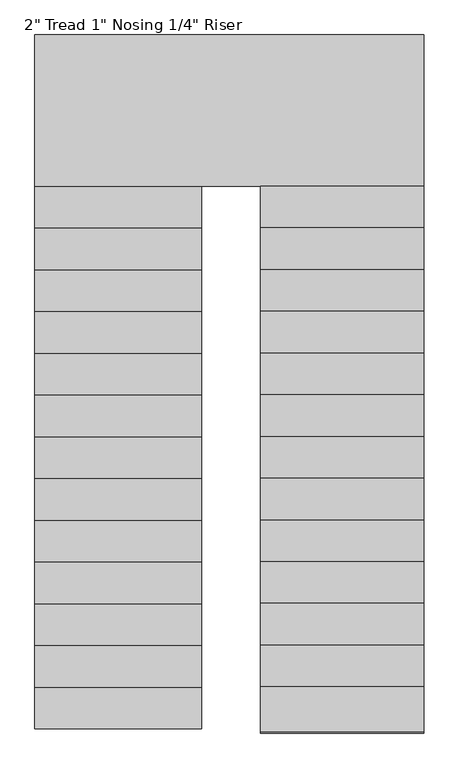
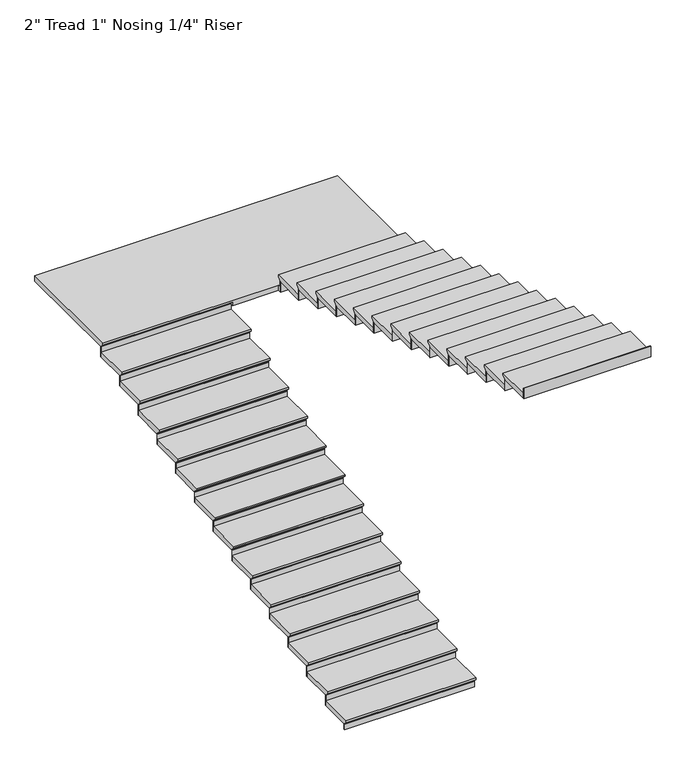
"""IFC4 building model written with IfcOpenShell, lengths in millimetres: stair flight geometry."""

from ifc_helpers import new_model, si_unit, origin, place, context, project, spatial, faceted_brep, source, transform, mapped, element, save


def stair_flight_b42c0417(model_context):
    return source(origin(), model_context, "Body", "Brep", [
        faceted_brep([(-629.5987998, 2564.5067329, 3284.7642857), (-629.5987998, 2564.5067329, 3303.8142857), (-1848.7987998, 2564.5067329, 3303.8142857), (-1848.7987998, 2564.5067329, 3284.7642857), (-629.5987998, 2589.9067329, 3259.3642857), (-1848.7987998, 2589.9067329, 3259.3642857), (-629.5987998, 2894.7067329, 3303.8142857), (-1848.7987998, 2894.7067329, 3303.8142857), (-1848.7987998, 2589.9067329, 3253.0142857), (-1848.7987998, 2894.7067329, 3253.0142857), (-629.5987998, 2894.7067329, 3253.0142857), (-629.5987998, 2589.9067329, 3253.0142857)], [[[0, 1, 2, 3]], [[4, 0, 3, 5]], [[2, 1, 6, 7]], [[8, 9, 10, 11]], [[2, 7, 9, 8, 5, 3]], [[8, 11, 4, 5]], [[6, 1, 0, 4, 11, 10]], [[7, 6, 10, 9]]]),
        faceted_brep([(-629.5987998, 2589.9067329, 3253.0142857), (-629.5987998, 2589.9067329, 3200.4), (-629.5987998, 2596.2567329, 3200.4), (-629.5987998, 2596.2567329, 3253.0142857), (-1848.7987998, 2589.9067329, 3253.0142857), (-1848.7987998, 2596.2567329, 3253.0142857), (-1848.7987998, 2596.2567329, 3200.4), (-1848.7987998, 2589.9067329, 3200.4)], [[[0, 1, 2, 3]], [[4, 5, 6, 7]], [[1, 0, 4, 7]], [[2, 1, 7, 6]], [[3, 2, 6, 5]], [[0, 3, 5, 4]]]),
        faceted_brep([(-629.5987998, 2894.7067329, 3356.4285714), (-629.5987998, 2894.7067329, 3253.0142857), (-629.5987998, 2901.0567329, 3253.0142857), (-629.5987998, 2901.0567329, 3356.4285714), (-1848.7987998, 2894.7067329, 3356.4285714), (-1848.7987998, 2901.0567329, 3356.4285714), (-1848.7987998, 2901.0567329, 3253.0142857), (-1848.7987998, 2894.7067329, 3253.0142857)], [[[0, 1, 2, 3]], [[4, 5, 6, 7]], [[1, 0, 4, 7]], [[2, 1, 7, 6]], [[3, 2, 6, 5]], [[0, 3, 5, 4]]]),
        faceted_brep([(-1848.7987998, 2869.3067329, 3407.2285714), (-629.5987998, 2869.3067329, 3407.2285714), (-629.5987998, 3199.5067329, 3407.2285714), (-1848.7987998, 3199.5067329, 3407.2285714), (-1848.7987998, 2894.7067329, 3356.4285714), (-1848.7987998, 3199.5067329, 3356.4285714), (-629.5987998, 3199.5067329, 3356.4285714), (-629.5987998, 2894.7067329, 3356.4285714), (-1848.7987998, 2894.7067329, 3362.7785714), (-1848.7987998, 2869.3067329, 3388.1785714), (-629.5987998, 2894.7067329, 3362.7785714), (-629.5987998, 2869.3067329, 3388.1785714)], [[[0, 1, 2, 3]], [[4, 5, 6, 7]], [[0, 3, 5, 4, 8, 9]], [[4, 7, 10, 8]], [[2, 1, 11, 10, 7, 6]], [[3, 2, 6, 5]], [[11, 1, 0, 9]], [[10, 11, 9, 8]]]),
        faceted_brep([(-629.5987998, 3199.5067329, 3459.8428571), (-629.5987998, 3199.5067329, 3356.4285714), (-629.5987998, 3205.8567329, 3356.4285714), (-629.5987998, 3205.8567329, 3459.8428571), (-1848.7987998, 3199.5067329, 3459.8428571), (-1848.7987998, 3205.8567329, 3459.8428571), (-1848.7987998, 3205.8567329, 3356.4285714), (-1848.7987998, 3199.5067329, 3356.4285714)], [[[0, 1, 2, 3]], [[4, 5, 6, 7]], [[1, 0, 4, 7]], [[2, 1, 7, 6]], [[3, 2, 6, 5]], [[0, 3, 5, 4]]]),
        faceted_brep([(-1848.7987998, 3174.1067329, 3510.6428571), (-629.5987998, 3174.1067329, 3510.6428571), (-629.5987998, 3504.3067329, 3510.6428571), (-1848.7987998, 3504.3067329, 3510.6428571), (-1848.7987998, 3199.5067329, 3459.8428571), (-1848.7987998, 3504.3067329, 3459.8428571), (-629.5987998, 3504.3067329, 3459.8428571), (-629.5987998, 3199.5067329, 3459.8428571), (-1848.7987998, 3199.5067329, 3466.1928571), (-1848.7987998, 3174.1067329, 3491.5928571), (-629.5987998, 3199.5067329, 3466.1928571), (-629.5987998, 3174.1067329, 3491.5928571)], [[[0, 1, 2, 3]], [[4, 5, 6, 7]], [[0, 3, 5, 4, 8, 9]], [[4, 7, 10, 8]], [[2, 1, 11, 10, 7, 6]], [[3, 2, 6, 5]], [[11, 1, 0, 9]], [[10, 11, 9, 8]]]),
        faceted_brep([(-629.5987998, 3504.3067329, 3563.2571429), (-629.5987998, 3504.3067329, 3459.8428571), (-629.5987998, 3510.6567329, 3459.8428571), (-629.5987998, 3510.6567329, 3563.2571429), (-1848.7987998, 3504.3067329, 3563.2571429), (-1848.7987998, 3510.6567329, 3563.2571429), (-1848.7987998, 3510.6567329, 3459.8428571), (-1848.7987998, 3504.3067329, 3459.8428571)], [[[0, 1, 2, 3]], [[4, 5, 6, 7]], [[1, 0, 4, 7]], [[2, 1, 7, 6]], [[3, 2, 6, 5]], [[0, 3, 5, 4]]]),
        faceted_brep([(-1848.7987998, 3478.9067329, 3614.0571429), (-629.5987998, 3478.9067329, 3614.0571429), (-629.5987998, 3809.1067329, 3614.0571429), (-1848.7987998, 3809.1067329, 3614.0571429), (-1848.7987998, 3504.3067329, 3563.2571429), (-1848.7987998, 3809.1067329, 3563.2571429), (-629.5987998, 3809.1067329, 3563.2571429), (-629.5987998, 3504.3067329, 3563.2571429), (-1848.7987998, 3504.3067329, 3569.6071429), (-1848.7987998, 3478.9067329, 3595.0071429), (-629.5987998, 3504.3067329, 3569.6071429), (-629.5987998, 3478.9067329, 3595.0071429)], [[[0, 1, 2, 3]], [[4, 5, 6, 7]], [[0, 3, 5, 4, 8, 9]], [[4, 7, 10, 8]], [[2, 1, 11, 10, 7, 6]], [[3, 2, 6, 5]], [[11, 1, 0, 9]], [[10, 11, 9, 8]]]),
        faceted_brep([(-629.5987998, 3809.1067329, 3666.6714286), (-629.5987998, 3809.1067329, 3563.2571429), (-629.5987998, 3815.4567329, 3563.2571429), (-629.5987998, 3815.4567329, 3666.6714286), (-1848.7987998, 3809.1067329, 3666.6714286), (-1848.7987998, 3815.4567329, 3666.6714286), (-1848.7987998, 3815.4567329, 3563.2571429), (-1848.7987998, 3809.1067329, 3563.2571429)], [[[0, 1, 2, 3]], [[4, 5, 6, 7]], [[1, 0, 4, 7]], [[2, 1, 7, 6]], [[3, 2, 6, 5]], [[0, 3, 5, 4]]]),
        faceted_brep([(-1848.7987998, 3783.7067329, 3717.4714286), (-629.5987998, 3783.7067329, 3717.4714286), (-629.5987998, 4113.9067329, 3717.4714286), (-1848.7987998, 4113.9067329, 3717.4714286), (-1848.7987998, 3809.1067329, 3666.6714286), (-1848.7987998, 4113.9067329, 3666.6714286), (-629.5987998, 4113.9067329, 3666.6714286), (-629.5987998, 3809.1067329, 3666.6714286), (-1848.7987998, 3809.1067329, 3673.0214286), (-1848.7987998, 3783.7067329, 3698.4214286), (-629.5987998, 3809.1067329, 3673.0214286), (-629.5987998, 3783.7067329, 3698.4214286)], [[[0, 1, 2, 3]], [[4, 5, 6, 7]], [[0, 3, 5, 4, 8, 9]], [[4, 7, 10, 8]], [[2, 1, 11, 10, 7, 6]], [[3, 2, 6, 5]], [[11, 1, 0, 9]], [[10, 11, 9, 8]]]),
        faceted_brep([(-629.5987998, 4113.9067329, 3770.0857143), (-629.5987998, 4113.9067329, 3666.6714286), (-629.5987998, 4120.2567329, 3666.6714286), (-629.5987998, 4120.2567329, 3770.0857143), (-1848.7987998, 4113.9067329, 3770.0857143), (-1848.7987998, 4120.2567329, 3770.0857143), (-1848.7987998, 4120.2567329, 3666.6714286), (-1848.7987998, 4113.9067329, 3666.6714286)], [[[0, 1, 2, 3]], [[4, 5, 6, 7]], [[1, 0, 4, 7]], [[2, 1, 7, 6]], [[3, 2, 6, 5]], [[0, 3, 5, 4]]]),
        faceted_brep([(-1848.7987998, 4088.5067329, 3820.8857143), (-629.5987998, 4088.5067329, 3820.8857143), (-629.5987998, 4418.7067329, 3820.8857143), (-1848.7987998, 4418.7067329, 3820.8857143), (-1848.7987998, 4113.9067329, 3770.0857143), (-1848.7987998, 4418.7067329, 3770.0857143), (-629.5987998, 4418.7067329, 3770.0857143), (-629.5987998, 4113.9067329, 3770.0857143), (-1848.7987998, 4113.9067329, 3776.4357143), (-1848.7987998, 4088.5067329, 3801.8357143), (-629.5987998, 4113.9067329, 3776.4357143), (-629.5987998, 4088.5067329, 3801.8357143)], [[[0, 1, 2, 3]], [[4, 5, 6, 7]], [[0, 3, 5, 4, 8, 9]], [[4, 7, 10, 8]], [[2, 1, 11, 10, 7, 6]], [[3, 2, 6, 5]], [[11, 1, 0, 9]], [[10, 11, 9, 8]]]),
        faceted_brep([(-629.5987998, 4418.7067329, 3873.5), (-629.5987998, 4418.7067329, 3770.0857143), (-629.5987998, 4425.0567329, 3770.0857143), (-629.5987998, 4425.0567329, 3873.5), (-1848.7987998, 4418.7067329, 3873.5), (-1848.7987998, 4425.0567329, 3873.5), (-1848.7987998, 4425.0567329, 3770.0857143), (-1848.7987998, 4418.7067329, 3770.0857143)], [[[0, 1, 2, 3]], [[4, 5, 6, 7]], [[1, 0, 4, 7]], [[2, 1, 7, 6]], [[3, 2, 6, 5]], [[0, 3, 5, 4]]]),
        faceted_brep([(-1848.7987998, 4393.3067329, 3924.3), (-629.5987998, 4393.3067329, 3924.3), (-629.5987998, 4723.5067329, 3924.3), (-1848.7987998, 4723.5067329, 3924.3), (-1848.7987998, 4418.7067329, 3873.5), (-1848.7987998, 4723.5067329, 3873.5), (-629.5987998, 4723.5067329, 3873.5), (-629.5987998, 4418.7067329, 3873.5), (-1848.7987998, 4418.7067329, 3879.85), (-1848.7987998, 4393.3067329, 3905.25), (-629.5987998, 4418.7067329, 3879.85), (-629.5987998, 4393.3067329, 3905.25)], [[[0, 1, 2, 3]], [[4, 5, 6, 7]], [[0, 3, 5, 4, 8, 9]], [[4, 7, 10, 8]], [[2, 1, 11, 10, 7, 6]], [[3, 2, 6, 5]], [[11, 1, 0, 9]], [[10, 11, 9, 8]]]),
        faceted_brep([(-629.5987998, 4723.5067329, 3976.9142857), (-629.5987998, 4723.5067329, 3873.5), (-629.5987998, 4729.8567329, 3873.5), (-629.5987998, 4729.8567329, 3976.9142857), (-1848.7987998, 4723.5067329, 3976.9142857), (-1848.7987998, 4729.8567329, 3976.9142857), (-1848.7987998, 4729.8567329, 3873.5), (-1848.7987998, 4723.5067329, 3873.5)], [[[0, 1, 2, 3]], [[4, 5, 6, 7]], [[1, 0, 4, 7]], [[2, 1, 7, 6]], [[3, 2, 6, 5]], [[0, 3, 5, 4]]]),
        faceted_brep([(-1848.7987998, 4698.1067329, 4027.7142857), (-629.5987998, 4698.1067329, 4027.7142857), (-629.5987998, 5028.3067329, 4027.7142857), (-1848.7987998, 5028.3067329, 4027.7142857), (-1848.7987998, 4723.5067329, 3976.9142857), (-1848.7987998, 5028.3067329, 3976.9142857), (-629.5987998, 5028.3067329, 3976.9142857), (-629.5987998, 4723.5067329, 3976.9142857), (-1848.7987998, 4723.5067329, 3983.2642857), (-1848.7987998, 4698.1067329, 4008.6642857), (-629.5987998, 4723.5067329, 3983.2642857), (-629.5987998, 4698.1067329, 4008.6642857)], [[[0, 1, 2, 3]], [[4, 5, 6, 7]], [[0, 3, 5, 4, 8, 9]], [[4, 7, 10, 8]], [[2, 1, 11, 10, 7, 6]], [[3, 2, 6, 5]], [[11, 1, 0, 9]], [[10, 11, 9, 8]]]),
        faceted_brep([(-629.5987998, 5028.3067329, 4080.3285714), (-629.5987998, 5028.3067329, 3976.9142857), (-629.5987998, 5034.6567329, 3976.9142857), (-629.5987998, 5034.6567329, 4080.3285714), (-1848.7987998, 5028.3067329, 4080.3285714), (-1848.7987998, 5034.6567329, 4080.3285714), (-1848.7987998, 5034.6567329, 3976.9142857), (-1848.7987998, 5028.3067329, 3976.9142857)], [[[0, 1, 2, 3]], [[4, 5, 6, 7]], [[1, 0, 4, 7]], [[2, 1, 7, 6]], [[3, 2, 6, 5]], [[0, 3, 5, 4]]]),
        faceted_brep([(-1848.7987998, 5002.9067329, 4131.1285714), (-629.5987998, 5002.9067329, 4131.1285714), (-629.5987998, 5333.1067329, 4131.1285714), (-1848.7987998, 5333.1067329, 4131.1285714), (-1848.7987998, 5028.3067329, 4080.3285714), (-1848.7987998, 5333.1067329, 4080.3285714), (-629.5987998, 5333.1067329, 4080.3285714), (-629.5987998, 5028.3067329, 4080.3285714), (-1848.7987998, 5028.3067329, 4086.6785714), (-1848.7987998, 5002.9067329, 4112.0785714), (-629.5987998, 5028.3067329, 4086.6785714), (-629.5987998, 5002.9067329, 4112.0785714)], [[[0, 1, 2, 3]], [[4, 5, 6, 7]], [[0, 3, 5, 4, 8, 9]], [[4, 7, 10, 8]], [[2, 1, 11, 10, 7, 6]], [[3, 2, 6, 5]], [[11, 1, 0, 9]], [[10, 11, 9, 8]]]),
        faceted_brep([(-629.5987998, 5333.1067329, 4183.7428571), (-629.5987998, 5333.1067329, 4080.3285714), (-629.5987998, 5339.4567329, 4080.3285714), (-629.5987998, 5339.4567329, 4183.7428571), (-1848.7987998, 5333.1067329, 4183.7428571), (-1848.7987998, 5339.4567329, 4183.7428571), (-1848.7987998, 5339.4567329, 4080.3285714), (-1848.7987998, 5333.1067329, 4080.3285714)], [[[0, 1, 2, 3]], [[4, 5, 6, 7]], [[1, 0, 4, 7]], [[2, 1, 7, 6]], [[3, 2, 6, 5]], [[0, 3, 5, 4]]]),
        faceted_brep([(-1848.7987998, 5307.7067329, 4234.5428571), (-629.5987998, 5307.7067329, 4234.5428571), (-629.5987998, 5637.9067329, 4234.5428571), (-1848.7987998, 5637.9067329, 4234.5428571), (-1848.7987998, 5333.1067329, 4183.7428571), (-1848.7987998, 5637.9067329, 4183.7428571), (-629.5987998, 5637.9067329, 4183.7428571), (-629.5987998, 5333.1067329, 4183.7428571), (-1848.7987998, 5333.1067329, 4190.0928571), (-1848.7987998, 5307.7067329, 4215.4928571), (-629.5987998, 5333.1067329, 4190.0928571), (-629.5987998, 5307.7067329, 4215.4928571)], [[[0, 1, 2, 3]], [[4, 5, 6, 7]], [[0, 3, 5, 4, 8, 9]], [[4, 7, 10, 8]], [[2, 1, 11, 10, 7, 6]], [[3, 2, 6, 5]], [[11, 1, 0, 9]], [[10, 11, 9, 8]]]),
        faceted_brep([(-629.5987998, 5637.9067329, 4287.1571429), (-629.5987998, 5637.9067329, 4183.7428571), (-629.5987998, 5644.2567329, 4183.7428571), (-629.5987998, 5644.2567329, 4287.1571429), (-1848.7987998, 5637.9067329, 4287.1571429), (-1848.7987998, 5644.2567329, 4287.1571429), (-1848.7987998, 5644.2567329, 4183.7428571), (-1848.7987998, 5637.9067329, 4183.7428571)], [[[0, 1, 2, 3]], [[4, 5, 6, 7]], [[1, 0, 4, 7]], [[2, 1, 7, 6]], [[3, 2, 6, 5]], [[0, 3, 5, 4]]]),
        faceted_brep([(-1848.7987998, 5612.5067329, 4337.9571429), (-629.5987998, 5612.5067329, 4337.9571429), (-629.5987998, 5942.7067329, 4337.9571429), (-1848.7987998, 5942.7067329, 4337.9571429), (-1848.7987998, 5637.9067329, 4287.1571429), (-1848.7987998, 5942.7067329, 4287.1571429), (-629.5987998, 5942.7067329, 4287.1571429), (-629.5987998, 5637.9067329, 4287.1571429), (-1848.7987998, 5637.9067329, 4293.5071429), (-1848.7987998, 5612.5067329, 4318.9071429), (-629.5987998, 5637.9067329, 4293.5071429), (-629.5987998, 5612.5067329, 4318.9071429)], [[[0, 1, 2, 3]], [[4, 5, 6, 7]], [[0, 3, 5, 4, 8, 9]], [[4, 7, 10, 8]], [[2, 1, 11, 10, 7, 6]], [[3, 2, 6, 5]], [[11, 1, 0, 9]], [[10, 11, 9, 8]]]),
        faceted_brep([(-629.5987998, 5942.7067329, 4390.5714286), (-629.5987998, 5942.7067329, 4287.1571429), (-629.5987998, 5949.0567329, 4287.1571429), (-629.5987998, 5949.0567329, 4390.5714286), (-1848.7987998, 5942.7067329, 4390.5714286), (-1848.7987998, 5949.0567329, 4390.5714286), (-1848.7987998, 5949.0567329, 4287.1571429), (-1848.7987998, 5942.7067329, 4287.1571429)], [[[0, 1, 2, 3]], [[4, 5, 6, 7]], [[1, 0, 4, 7]], [[2, 1, 7, 6]], [[3, 2, 6, 5]], [[0, 3, 5, 4]]]),
        faceted_brep([(-1848.7987998, 5917.3067329, 4441.3714286), (-629.5987998, 5917.3067329, 4441.3714286), (-629.5987998, 6247.5067329, 4441.3714286), (-1848.7987998, 6247.5067329, 4441.3714286), (-1848.7987998, 5942.7067329, 4390.5714286), (-1848.7987998, 6247.5067329, 4390.5714286), (-629.5987998, 6247.5067329, 4390.5714286), (-629.5987998, 5942.7067329, 4390.5714286), (-1848.7987998, 5942.7067329, 4396.9214286), (-1848.7987998, 5917.3067329, 4422.3214286), (-629.5987998, 5942.7067329, 4396.9214286), (-629.5987998, 5917.3067329, 4422.3214286)], [[[0, 1, 2, 3]], [[4, 5, 6, 7]], [[0, 3, 5, 4, 8, 9]], [[4, 7, 10, 8]], [[2, 1, 11, 10, 7, 6]], [[3, 2, 6, 5]], [[11, 1, 0, 9]], [[10, 11, 9, 8]]]),
        faceted_brep([(-629.5987998, 6247.5067329, 4493.9857143), (-629.5987998, 6247.5067329, 4390.5714286), (-629.5987998, 6253.8567329, 4390.5714286), (-629.5987998, 6253.8567329, 4493.9857143), (-1848.7987998, 6247.5067329, 4493.9857143), (-1848.7987998, 6253.8567329, 4493.9857143), (-1848.7987998, 6253.8567329, 4390.5714286), (-1848.7987998, 6247.5067329, 4390.5714286)], [[[0, 1, 2, 3]], [[4, 5, 6, 7]], [[1, 0, 4, 7]], [[2, 1, 7, 6]], [[3, 2, 6, 5]], [[0, 3, 5, 4]]]),
        faceted_brep([(-1848.7987998, 6222.1067329, 4544.7857143), (-629.5987998, 6222.1067329, 4544.7857143), (-629.5987998, 6552.3067329, 4544.7857143), (-1848.7987998, 6552.3067329, 4544.7857143), (-1848.7987998, 6247.5067329, 4493.9857143), (-1848.7987998, 6552.3067329, 4493.9857143), (-629.5987998, 6552.3067329, 4493.9857143), (-629.5987998, 6247.5067329, 4493.9857143), (-1848.7987998, 6247.5067329, 4500.3357143), (-1848.7987998, 6222.1067329, 4525.7357143), (-629.5987998, 6247.5067329, 4500.3357143), (-629.5987998, 6222.1067329, 4525.7357143)], [[[0, 1, 2, 3]], [[4, 5, 6, 7]], [[0, 3, 5, 4, 8, 9]], [[4, 7, 10, 8]], [[2, 1, 11, 10, 7, 6]], [[3, 2, 6, 5]], [[11, 1, 0, 9]], [[10, 11, 9, 8]]]),
        faceted_brep([(-629.5987998, 6552.3067329, 4597.4), (-629.5987998, 6552.3067329, 4493.9857143), (-629.5987998, 6558.6567329, 4493.9857143), (-629.5987998, 6558.6567329, 4597.4), (-1848.7987998, 6552.3067329, 4597.4), (-1848.7987998, 6558.6567329, 4597.4), (-1848.7987998, 6558.6567329, 4493.9857143), (-1848.7987998, 6552.3067329, 4493.9857143)], [[[0, 1, 2, 3]], [[4, 5, 6, 7]], [[1, 0, 4, 7]], [[2, 1, 7, 6]], [[3, 2, 6, 5]], [[0, 3, 5, 4]]]),
        faceted_brep([(996.0012002, 6501.5067329, 4648.2), (996.0012002, 7631.8067329, 4648.2), (-1848.7987998, 7631.8067329, 4648.2), (-1848.7987998, 6526.9067329, 4648.2), (-197.7987915, 6526.9067329, 4648.2), (-197.7987915, 6501.5067329, 4648.2), (996.0012002, 7631.8067329, 4597.4), (996.0012002, 6501.5067329, 4597.4), (-197.7987915, 6501.5067329, 4597.4), (-197.7987915, 6526.9067329, 4597.4), (-629.5987998, 6526.9067329, 4597.4), (-629.5987998, 6552.3067329, 4597.4), (-1848.7987998, 6552.3067329, 4597.4), (-1848.7987998, 7631.8067329, 4597.4), (-629.5987998, 6552.3067329, 4603.75), (-1848.7987998, 6552.3067329, 4603.75), (-1848.7987998, 6526.9067329, 4629.15), (-629.5987998, 6526.9067329, 4629.15)], [[[0, 1, 2, 3, 4, 5]], [[6, 7, 8, 9, 10, 11, 12, 13]], [[1, 0, 7, 6]], [[2, 1, 6, 13]], [[12, 11, 14, 15]], [[4, 3, 16, 17, 10, 9]], [[5, 4, 9, 8]], [[0, 5, 8, 7]], [[16, 15, 14, 17]], [[3, 2, 13, 12, 15, 16]], [[11, 10, 17, 14]]]),
        faceted_brep([(-197.7987915, 6501.5067329, 4700.8142857), (-197.7987915, 6501.5067329, 4597.4), (-197.7987915, 6495.1567329, 4597.4), (-197.7987915, 6495.1567329, 4700.8142857), (996.0012002, 6501.5067329, 4700.8142857), (996.0012002, 6495.1567329, 4700.8142857), (996.0012002, 6495.1567329, 4597.4), (996.0012002, 6501.5067329, 4597.4)], [[[0, 1, 2, 3]], [[4, 5, 6, 7]], [[1, 0, 4, 7]], [[2, 1, 7, 6]], [[3, 2, 6, 5]], [[0, 3, 5, 4]]]),
        faceted_brep([(996.0012002, 6526.9067329, 4751.6142857), (-197.7987915, 6526.9067329, 4751.6142857), (-197.7987915, 6196.7067329, 4751.6142857), (996.0012002, 6196.7067329, 4751.6142857), (996.0012002, 6501.5067329, 4700.8142857), (996.0012002, 6196.7067329, 4700.8142857), (-197.7987915, 6196.7067329, 4700.8142857), (-197.7987915, 6501.5067329, 4700.8142857), (996.0012002, 6501.5067329, 4707.1642857), (996.0012002, 6526.9067329, 4732.5642857), (-197.7987915, 6501.5067329, 4707.1642857), (-197.7987915, 6526.9067329, 4732.5642857)], [[[0, 1, 2, 3]], [[4, 5, 6, 7]], [[0, 3, 5, 4, 8, 9]], [[4, 7, 10, 8]], [[2, 1, 11, 10, 7, 6]], [[3, 2, 6, 5]], [[11, 1, 0, 9]], [[10, 11, 9, 8]]]),
        faceted_brep([(-197.7987915, 6196.7067329, 4804.2285714), (-197.7987915, 6196.7067329, 4700.8142857), (-197.7987915, 6190.3567329, 4700.8142857), (-197.7987915, 6190.3567329, 4804.2285714), (996.0012002, 6196.7067329, 4804.2285714), (996.0012002, 6190.3567329, 4804.2285714), (996.0012002, 6190.3567329, 4700.8142857), (996.0012002, 6196.7067329, 4700.8142857)], [[[0, 1, 2, 3]], [[4, 5, 6, 7]], [[1, 0, 4, 7]], [[2, 1, 7, 6]], [[3, 2, 6, 5]], [[0, 3, 5, 4]]]),
        faceted_brep([(996.0012002, 6222.1067329, 4855.0285714), (-197.7987915, 6222.1067329, 4855.0285714), (-197.7987915, 5891.9067329, 4855.0285714), (996.0012002, 5891.9067329, 4855.0285714), (996.0012002, 6196.7067329, 4804.2285714), (996.0012002, 5891.9067329, 4804.2285714), (-197.7987915, 5891.9067329, 4804.2285714), (-197.7987915, 6196.7067329, 4804.2285714), (996.0012002, 6196.7067329, 4810.5785714), (996.0012002, 6222.1067329, 4835.9785714), (-197.7987915, 6196.7067329, 4810.5785714), (-197.7987915, 6222.1067329, 4835.9785714)], [[[0, 1, 2, 3]], [[4, 5, 6, 7]], [[0, 3, 5, 4, 8, 9]], [[4, 7, 10, 8]], [[2, 1, 11, 10, 7, 6]], [[3, 2, 6, 5]], [[11, 1, 0, 9]], [[10, 11, 9, 8]]]),
        faceted_brep([(-197.7987915, 5891.9067329, 4907.6428571), (-197.7987915, 5891.9067329, 4804.2285714), (-197.7987915, 5885.5567329, 4804.2285714), (-197.7987915, 5885.5567329, 4907.6428571), (996.0012002, 5891.9067329, 4907.6428571), (996.0012002, 5885.5567329, 4907.6428571), (996.0012002, 5885.5567329, 4804.2285714), (996.0012002, 5891.9067329, 4804.2285714)], [[[0, 1, 2, 3]], [[4, 5, 6, 7]], [[1, 0, 4, 7]], [[2, 1, 7, 6]], [[3, 2, 6, 5]], [[0, 3, 5, 4]]]),
        faceted_brep([(996.0012002, 5917.3067329, 4958.4428571), (-197.7987915, 5917.3067329, 4958.4428571), (-197.7987915, 5587.1067329, 4958.4428571), (996.0012002, 5587.1067329, 4958.4428571), (996.0012002, 5891.9067329, 4907.6428571), (996.0012002, 5587.1067329, 4907.6428571), (-197.7987915, 5587.1067329, 4907.6428571), (-197.7987915, 5891.9067329, 4907.6428571), (996.0012002, 5891.9067329, 4913.9928571), (996.0012002, 5917.3067329, 4939.3928571), (-197.7987915, 5891.9067329, 4913.9928571), (-197.7987915, 5917.3067329, 4939.3928571)], [[[0, 1, 2, 3]], [[4, 5, 6, 7]], [[0, 3, 5, 4, 8, 9]], [[4, 7, 10, 8]], [[2, 1, 11, 10, 7, 6]], [[3, 2, 6, 5]], [[11, 1, 0, 9]], [[10, 11, 9, 8]]]),
        faceted_brep([(-197.7987915, 5587.1067329, 5011.0571429), (-197.7987915, 5587.1067329, 4907.6428571), (-197.7987915, 5580.7567329, 4907.6428571), (-197.7987915, 5580.7567329, 5011.0571429), (996.0012002, 5587.1067329, 5011.0571429), (996.0012002, 5580.7567329, 5011.0571429), (996.0012002, 5580.7567329, 4907.6428571), (996.0012002, 5587.1067329, 4907.6428571)], [[[0, 1, 2, 3]], [[4, 5, 6, 7]], [[1, 0, 4, 7]], [[2, 1, 7, 6]], [[3, 2, 6, 5]], [[0, 3, 5, 4]]]),
        faceted_brep([(996.0012002, 5612.5067329, 5061.8571429), (-197.7987915, 5612.5067329, 5061.8571429), (-197.7987915, 5282.3067329, 5061.8571429), (996.0012002, 5282.3067329, 5061.8571429), (996.0012002, 5587.1067329, 5011.0571429), (996.0012002, 5282.3067329, 5011.0571429), (-197.7987915, 5282.3067329, 5011.0571429), (-197.7987915, 5587.1067329, 5011.0571429), (996.0012002, 5587.1067329, 5017.4071429), (996.0012002, 5612.5067329, 5042.8071429), (-197.7987915, 5587.1067329, 5017.4071429), (-197.7987915, 5612.5067329, 5042.8071429)], [[[0, 1, 2, 3]], [[4, 5, 6, 7]], [[0, 3, 5, 4, 8, 9]], [[4, 7, 10, 8]], [[2, 1, 11, 10, 7, 6]], [[3, 2, 6, 5]], [[11, 1, 0, 9]], [[10, 11, 9, 8]]]),
        faceted_brep([(-197.7987915, 5282.3067329, 5114.4714286), (-197.7987915, 5282.3067329, 5011.0571429), (-197.7987915, 5275.9567329, 5011.0571429), (-197.7987915, 5275.9567329, 5114.4714286), (996.0012002, 5282.3067329, 5114.4714286), (996.0012002, 5275.9567329, 5114.4714286), (996.0012002, 5275.9567329, 5011.0571429), (996.0012002, 5282.3067329, 5011.0571429)], [[[0, 1, 2, 3]], [[4, 5, 6, 7]], [[1, 0, 4, 7]], [[2, 1, 7, 6]], [[3, 2, 6, 5]], [[0, 3, 5, 4]]]),
        faceted_brep([(996.0012002, 5307.7067329, 5165.2714286), (-197.7987915, 5307.7067329, 5165.2714286), (-197.7987915, 4977.5067329, 5165.2714286), (996.0012002, 4977.5067329, 5165.2714286), (996.0012002, 5282.3067329, 5114.4714286), (996.0012002, 4977.5067329, 5114.4714286), (-197.7987915, 4977.5067329, 5114.4714286), (-197.7987915, 5282.3067329, 5114.4714286), (996.0012002, 5282.3067329, 5120.8214286), (996.0012002, 5307.7067329, 5146.2214286), (-197.7987915, 5282.3067329, 5120.8214286), (-197.7987915, 5307.7067329, 5146.2214286)], [[[0, 1, 2, 3]], [[4, 5, 6, 7]], [[0, 3, 5, 4, 8, 9]], [[4, 7, 10, 8]], [[2, 1, 11, 10, 7, 6]], [[3, 2, 6, 5]], [[11, 1, 0, 9]], [[10, 11, 9, 8]]]),
        faceted_brep([(-197.7987915, 4977.5067329, 5217.8857143), (-197.7987915, 4977.5067329, 5114.4714286), (-197.7987915, 4971.1567329, 5114.4714286), (-197.7987915, 4971.1567329, 5217.8857143), (996.0012002, 4977.5067329, 5217.8857143), (996.0012002, 4971.1567329, 5217.8857143), (996.0012002, 4971.1567329, 5114.4714286), (996.0012002, 4977.5067329, 5114.4714286)], [[[0, 1, 2, 3]], [[4, 5, 6, 7]], [[1, 0, 4, 7]], [[2, 1, 7, 6]], [[3, 2, 6, 5]], [[0, 3, 5, 4]]]),
        faceted_brep([(996.0012002, 5002.9067329, 5268.6857143), (-197.7987915, 5002.9067329, 5268.6857143), (-197.7987915, 4672.7067329, 5268.6857143), (996.0012002, 4672.7067329, 5268.6857143), (996.0012002, 4977.5067329, 5217.8857143), (996.0012002, 4672.7067329, 5217.8857143), (-197.7987915, 4672.7067329, 5217.8857143), (-197.7987915, 4977.5067329, 5217.8857143), (996.0012002, 4977.5067329, 5224.2357143), (996.0012002, 5002.9067329, 5249.6357143), (-197.7987915, 4977.5067329, 5224.2357143), (-197.7987915, 5002.9067329, 5249.6357143)], [[[0, 1, 2, 3]], [[4, 5, 6, 7]], [[0, 3, 5, 4, 8, 9]], [[4, 7, 10, 8]], [[2, 1, 11, 10, 7, 6]], [[3, 2, 6, 5]], [[11, 1, 0, 9]], [[10, 11, 9, 8]]]),
        faceted_brep([(-197.7987915, 4672.7067329, 5321.3), (-197.7987915, 4672.7067329, 5217.8857143), (-197.7987915, 4666.3567329, 5217.8857143), (-197.7987915, 4666.3567329, 5321.3), (996.0012002, 4672.7067329, 5321.3), (996.0012002, 4666.3567329, 5321.3), (996.0012002, 4666.3567329, 5217.8857143), (996.0012002, 4672.7067329, 5217.8857143)], [[[0, 1, 2, 3]], [[4, 5, 6, 7]], [[1, 0, 4, 7]], [[2, 1, 7, 6]], [[3, 2, 6, 5]], [[0, 3, 5, 4]]]),
        faceted_brep([(996.0012002, 4698.1067329, 5372.1), (-197.7987915, 4698.1067329, 5372.1), (-197.7987915, 4367.9067329, 5372.1), (996.0012002, 4367.9067329, 5372.1), (996.0012002, 4672.7067329, 5321.3), (996.0012002, 4367.9067329, 5321.3), (-197.7987915, 4367.9067329, 5321.3), (-197.7987915, 4672.7067329, 5321.3), (996.0012002, 4672.7067329, 5327.65), (996.0012002, 4698.1067329, 5353.05), (-197.7987915, 4672.7067329, 5327.65), (-197.7987915, 4698.1067329, 5353.05)], [[[0, 1, 2, 3]], [[4, 5, 6, 7]], [[0, 3, 5, 4, 8, 9]], [[4, 7, 10, 8]], [[2, 1, 11, 10, 7, 6]], [[3, 2, 6, 5]], [[11, 1, 0, 9]], [[10, 11, 9, 8]]]),
        faceted_brep([(-197.7987915, 4367.9067329, 5424.7142857), (-197.7987915, 4367.9067329, 5321.3), (-197.7987915, 4361.5567329, 5321.3), (-197.7987915, 4361.5567329, 5424.7142857), (996.0012002, 4367.9067329, 5424.7142857), (996.0012002, 4361.5567329, 5424.7142857), (996.0012002, 4361.5567329, 5321.3), (996.0012002, 4367.9067329, 5321.3)], [[[0, 1, 2, 3]], [[4, 5, 6, 7]], [[1, 0, 4, 7]], [[2, 1, 7, 6]], [[3, 2, 6, 5]], [[0, 3, 5, 4]]]),
        faceted_brep([(996.0012002, 4393.3067329, 5475.5142857), (-197.7987915, 4393.3067329, 5475.5142857), (-197.7987915, 4063.1067329, 5475.5142857), (996.0012002, 4063.1067329, 5475.5142857), (996.0012002, 4367.9067329, 5424.7142857), (996.0012002, 4063.1067329, 5424.7142857), (-197.7987915, 4063.1067329, 5424.7142857), (-197.7987915, 4367.9067329, 5424.7142857), (996.0012002, 4367.9067329, 5431.0642857), (996.0012002, 4393.3067329, 5456.4642857), (-197.7987915, 4367.9067329, 5431.0642857), (-197.7987915, 4393.3067329, 5456.4642857)], [[[0, 1, 2, 3]], [[4, 5, 6, 7]], [[0, 3, 5, 4, 8, 9]], [[4, 7, 10, 8]], [[2, 1, 11, 10, 7, 6]], [[3, 2, 6, 5]], [[11, 1, 0, 9]], [[10, 11, 9, 8]]]),
        faceted_brep([(-197.7987915, 4063.1067329, 5528.1285714), (-197.7987915, 4063.1067329, 5424.7142857), (-197.7987915, 4056.7567329, 5424.7142857), (-197.7987915, 4056.7567329, 5528.1285714), (996.0012002, 4063.1067329, 5528.1285714), (996.0012002, 4056.7567329, 5528.1285714), (996.0012002, 4056.7567329, 5424.7142857), (996.0012002, 4063.1067329, 5424.7142857)], [[[0, 1, 2, 3]], [[4, 5, 6, 7]], [[1, 0, 4, 7]], [[2, 1, 7, 6]], [[3, 2, 6, 5]], [[0, 3, 5, 4]]]),
        faceted_brep([(996.0012002, 4088.5067329, 5578.9285714), (-197.7987915, 4088.5067329, 5578.9285714), (-197.7987915, 3758.3067329, 5578.9285714), (996.0012002, 3758.3067329, 5578.9285714), (996.0012002, 4063.1067329, 5528.1285714), (996.0012002, 3758.3067329, 5528.1285714), (-197.7987915, 3758.3067329, 5528.1285714), (-197.7987915, 4063.1067329, 5528.1285714), (996.0012002, 4063.1067329, 5534.4785714), (996.0012002, 4088.5067329, 5559.8785714), (-197.7987915, 4063.1067329, 5534.4785714), (-197.7987915, 4088.5067329, 5559.8785714)], [[[0, 1, 2, 3]], [[4, 5, 6, 7]], [[0, 3, 5, 4, 8, 9]], [[4, 7, 10, 8]], [[2, 1, 11, 10, 7, 6]], [[3, 2, 6, 5]], [[11, 1, 0, 9]], [[10, 11, 9, 8]]]),
        faceted_brep([(-197.7987915, 3758.3067329, 5631.5428571), (-197.7987915, 3758.3067329, 5528.1285714), (-197.7987915, 3751.9567329, 5528.1285714), (-197.7987915, 3751.9567329, 5631.5428571), (996.0012002, 3758.3067329, 5631.5428571), (996.0012002, 3751.9567329, 5631.5428571), (996.0012002, 3751.9567329, 5528.1285714), (996.0012002, 3758.3067329, 5528.1285714)], [[[0, 1, 2, 3]], [[4, 5, 6, 7]], [[1, 0, 4, 7]], [[2, 1, 7, 6]], [[3, 2, 6, 5]], [[0, 3, 5, 4]]]),
        faceted_brep([(996.0012002, 3783.7067329, 5682.3428571), (-197.7987915, 3783.7067329, 5682.3428571), (-197.7987915, 3453.5067329, 5682.3428571), (996.0012002, 3453.5067329, 5682.3428571), (996.0012002, 3758.3067329, 5631.5428571), (996.0012002, 3453.5067329, 5631.5428571), (-197.7987915, 3453.5067329, 5631.5428571), (-197.7987915, 3758.3067329, 5631.5428571), (996.0012002, 3758.3067329, 5637.8928571), (996.0012002, 3783.7067329, 5663.2928571), (-197.7987915, 3758.3067329, 5637.8928571), (-197.7987915, 3783.7067329, 5663.2928571)], [[[0, 1, 2, 3]], [[4, 5, 6, 7]], [[0, 3, 5, 4, 8, 9]], [[4, 7, 10, 8]], [[2, 1, 11, 10, 7, 6]], [[3, 2, 6, 5]], [[11, 1, 0, 9]], [[10, 11, 9, 8]]]),
        faceted_brep([(-197.7987915, 3453.5067329, 5734.9571429), (-197.7987915, 3453.5067329, 5631.5428571), (-197.7987915, 3447.1567329, 5631.5428571), (-197.7987915, 3447.1567329, 5734.9571429), (996.0012002, 3453.5067329, 5734.9571429), (996.0012002, 3447.1567329, 5734.9571429), (996.0012002, 3447.1567329, 5631.5428571), (996.0012002, 3453.5067329, 5631.5428571)], [[[0, 1, 2, 3]], [[4, 5, 6, 7]], [[1, 0, 4, 7]], [[2, 1, 7, 6]], [[3, 2, 6, 5]], [[0, 3, 5, 4]]]),
        faceted_brep([(996.0012002, 3478.9067329, 5785.7571429), (-197.7987915, 3478.9067329, 5785.7571429), (-197.7987915, 3148.7067329, 5785.7571429), (996.0012002, 3148.7067329, 5785.7571429), (996.0012002, 3453.5067329, 5734.9571429), (996.0012002, 3148.7067329, 5734.9571429), (-197.7987915, 3148.7067329, 5734.9571429), (-197.7987915, 3453.5067329, 5734.9571429), (996.0012002, 3453.5067329, 5741.3071429), (996.0012002, 3478.9067329, 5766.7071429), (-197.7987915, 3453.5067329, 5741.3071429), (-197.7987915, 3478.9067329, 5766.7071429)], [[[0, 1, 2, 3]], [[4, 5, 6, 7]], [[0, 3, 5, 4, 8, 9]], [[4, 7, 10, 8]], [[2, 1, 11, 10, 7, 6]], [[3, 2, 6, 5]], [[11, 1, 0, 9]], [[10, 11, 9, 8]]]),
        faceted_brep([(-197.7987915, 3148.7067329, 5838.3714286), (-197.7987915, 3148.7067329, 5734.9571429), (-197.7987915, 3142.3567329, 5734.9571429), (-197.7987915, 3142.3567329, 5838.3714286), (996.0012002, 3148.7067329, 5838.3714286), (996.0012002, 3142.3567329, 5838.3714286), (996.0012002, 3142.3567329, 5734.9571429), (996.0012002, 3148.7067329, 5734.9571429)], [[[0, 1, 2, 3]], [[4, 5, 6, 7]], [[1, 0, 4, 7]], [[2, 1, 7, 6]], [[3, 2, 6, 5]], [[0, 3, 5, 4]]]),
        faceted_brep([(996.0012002, 3174.1067329, 5889.1714286), (-197.7987915, 3174.1067329, 5889.1714286), (-197.7987915, 2843.9067329, 5889.1714286), (996.0012002, 2843.9067329, 5889.1714286), (996.0012002, 3148.7067329, 5838.3714286), (996.0012002, 2843.9067329, 5838.3714286), (-197.7987915, 2843.9067329, 5838.3714286), (-197.7987915, 3148.7067329, 5838.3714286), (996.0012002, 3148.7067329, 5844.7214286), (996.0012002, 3174.1067329, 5870.1214286), (-197.7987915, 3148.7067329, 5844.7214286), (-197.7987915, 3174.1067329, 5870.1214286)], [[[0, 1, 2, 3]], [[4, 5, 6, 7]], [[0, 3, 5, 4, 8, 9]], [[4, 7, 10, 8]], [[2, 1, 11, 10, 7, 6]], [[3, 2, 6, 5]], [[11, 1, 0, 9]], [[10, 11, 9, 8]]]),
        faceted_brep([(-197.7987915, 2843.9067329, 5941.7857143), (-197.7987915, 2843.9067329, 5838.3714286), (-197.7987915, 2837.5567329, 5838.3714286), (-197.7987915, 2837.5567329, 5941.7857143), (996.0012002, 2843.9067329, 5941.7857143), (996.0012002, 2837.5567329, 5941.7857143), (996.0012002, 2837.5567329, 5838.3714286), (996.0012002, 2843.9067329, 5838.3714286)], [[[0, 1, 2, 3]], [[4, 5, 6, 7]], [[1, 0, 4, 7]], [[2, 1, 7, 6]], [[3, 2, 6, 5]], [[0, 3, 5, 4]]]),
        faceted_brep([(-197.7987915, 2539.1067329, 6045.2), (-197.7987915, 2539.1067329, 5941.7857143), (-197.7987915, 2532.7567329, 5941.7857143), (-197.7987915, 2532.7567329, 6045.2), (996.0012002, 2539.1067329, 6045.2), (996.0012002, 2532.7567329, 6045.2), (996.0012002, 2532.7567329, 5941.7857143), (996.0012002, 2539.1067329, 5941.7857143)], [[[0, 1, 2, 3]], [[4, 5, 6, 7]], [[1, 0, 4, 7]], [[2, 1, 7, 6]], [[3, 2, 6, 5]], [[0, 3, 5, 4]]]),
        faceted_brep([(996.0012002, 2869.3067329, 5992.5857143), (-197.7987915, 2869.3067329, 5992.5857143), (-197.7987915, 2539.1067329, 5992.5857143), (996.0012002, 2539.1067329, 5992.5857143), (996.0012002, 2843.9067329, 5941.7857143), (996.0012002, 2539.1067329, 5941.7857143), (-197.7987915, 2539.1067329, 5941.7857143), (-197.7987915, 2843.9067329, 5941.7857143), (996.0012002, 2843.9067329, 5948.1357143), (996.0012002, 2869.3067329, 5973.5357143), (-197.7987915, 2843.9067329, 5948.1357143), (-197.7987915, 2869.3067329, 5973.5357143)], [[[0, 1, 2, 3]], [[4, 5, 6, 7]], [[0, 3, 5, 4, 8, 9]], [[4, 7, 10, 8]], [[2, 1, 11, 10, 7, 6]], [[3, 2, 6, 5]], [[11, 1, 0, 9]], [[10, 11, 9, 8]]]),
    ])


if __name__ == "__main__":
    model = new_model("IFC4")
    model_context = context("Model", 3, world=origin())
    ifc_project = project(units=[si_unit("LENGTHUNIT", "METRE", prefix="MILLI")], contexts=[model_context])
    site = spatial("IfcSite", under=ifc_project)
    building = spatial("IfcBuilding", under=site)
    placement = place(None, origin())
    stair_flight_shape = stair_flight_b42c0417(model_context)
    element("IfcStairFlight", 1, ObjectType="2\" Tread 1\" Nosing 1/4\" Riser", at=placement, inside=building, context=model_context, shape_type="MappedRepresentation", body=[
        mapped(stair_flight_shape, transform((0.0, 0.0, 0.0), x_axis=(1.0, 0.0, 0.0), y_axis=(0.0, 1.0, 0.0), z_axis=(0.0, 0.0, 1.0))),
    ])
    save(model, "model.ifc")
